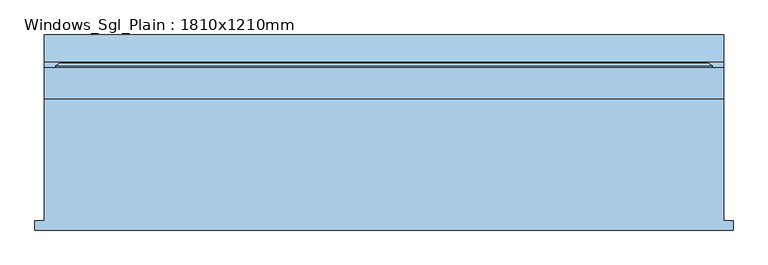
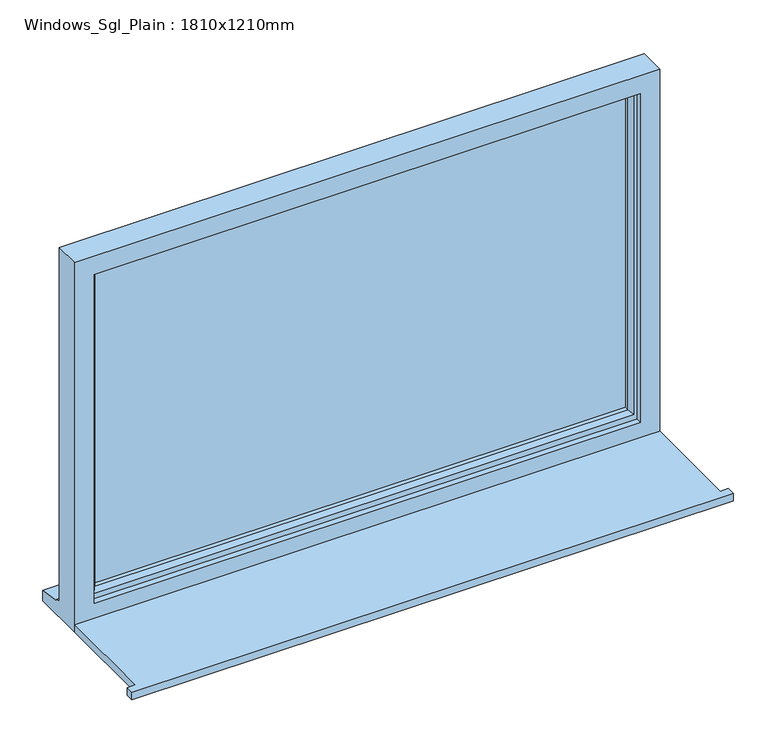
"""IFC4 building model written with IfcOpenShell, lengths in millimetres: window geometry, Windows_Sgl_Plain : 1810x1210mm."""

from ifc_helpers import new_model, si_unit, frame, origin, place, context, project, spatial, polyline, outline, extrude, faceted_brep, source, transform, mapped, element, save


def windows_sgl_plain_1810x1210mm_33e58113(model_context):
    return source(origin(), model_context, "Body", "SolidModel", [
        extrude(outline(polyline([(-930.0, -245.1434322), (-930.0, -220.1434322), (-905.0, -220.1434322), (-905.0, 104.0565678), (905.0, 104.0565678), (905.0, -220.1434322), (930.0, -220.1434322), (930.0, -245.1434322), (-930.0, -245.1434322)])), frame((0.0, 0.0, 900.0), z_axis=(0.0, 0.0, 1.0), x_axis=(1.0, 0.0, 0.0)), (0.0, 0.0, 1.0), 25.0),
        faceted_brep([(-905.0, 104.0565678, 900.0), (905.0, 104.0565678, 900.0), (905.0, 104.0565678, 2110.0), (-905.0, 104.0565678, 2110.0), (-845.0, 104.0565678, 2050.0), (845.0, 104.0565678, 2050.0), (845.0, 104.0565678, 975.0), (-845.0, 104.0565678, 975.0), (-905.0, 187.0565678, 2110.0), (-905.0, 187.0565678, 951.0), (-905.0, 202.0565678, 949.68767), (-905.0, 202.0565678, 944.7449676), (-905.0, 274.5565678, 933.8088847), (-905.0, 274.5565678, 900.0), (905.0, 187.0565678, 2110.0), (905.0, 187.0565678, 951.0), (-865.0, 187.0565678, 2070.0), (-865.0, 187.0565678, 963.0), (865.0, 187.0565678, 963.0), (865.0, 187.0565678, 2070.0), (-865.0, 122.0565678, 2070.0), (-865.0, 122.0565678, 963.0), (865.0, 122.0565678, 2070.0), (865.0, 122.0565678, 963.0), (-845.0, 122.0565678, 2050.0), (-845.0, 122.0565678, 975.0), (845.0, 122.0565678, 975.0), (845.0, 122.0565678, 2050.0), (905.0, 274.5565678, 900.0), (905.0, 274.5565678, 933.8088847), (905.0, 202.0565678, 944.7449676), (905.0, 202.0565678, 949.68767)], [[[0, 1, 2, 3], [4, 5, 6, 7]], [[0, 3, 8, 9, 10, 11, 12, 13]], [[9, 8, 14, 15], [16, 17, 18, 19]], [[17, 16, 20, 21]], [[20, 22, 23, 21], [24, 25, 26, 27]], [[24, 4, 7, 25]], [[3, 2, 14, 8]], [[16, 19, 22, 20]], [[5, 4, 24, 27]], [[15, 14, 2, 1, 28, 29, 30, 31]], [[19, 18, 23, 22]], [[5, 27, 26, 6]], [[28, 1, 0, 13]], [[29, 28, 13, 12]], [[30, 29, 12, 11]], [[31, 30, 11, 10]], [[15, 31, 10, 9]], [[21, 23, 18, 17]], [[7, 6, 26, 25]]]),
        extrude(outline(polyline([(835.0, 151.0565678), (-835.0, 151.0565678), (-835.0, 175.0565678), (835.0, 175.0565678), (835.0, 151.0565678)])), frame((0.0, 0.0, 993.0), z_axis=(0.0, 0.0, 1.0), x_axis=(1.0, 0.0, 0.0)), (0.0, 0.0, 1.0), 1047.0),
        faceted_brep([(-875.0, 187.0565678, 2080.0), (-875.0, 192.8300705, 2080.0), (-875.0, 192.8300705, 953.0), (-875.0, 187.0565678, 953.0), (-865.0, 122.0565678, 2070.0), (-865.0, 187.0565678, 2070.0), (-865.0, 187.0565678, 963.0), (-865.0, 122.0565678, 963.0), (-825.0, 136.5494677, 2030.0), (-835.1480377, 122.0565678, 2040.1480377), (-835.1480377, 122.0565678, 992.8519623), (-825.0, 136.5494677, 1003.0), (-825.0, 151.0565678, 2030.0), (-825.0, 151.0565678, 1003.0), (-835.0, 175.0565678, 2040.0), (-835.0, 151.0565678, 2040.0), (-835.0, 151.0565678, 993.0), (-835.0, 175.0565678, 993.0), (-825.0, 192.8300705, 2030.0), (-825.0, 175.0565678, 2030.0), (-825.0, 175.0565678, 1003.0), (-825.0, 192.8300705, 1003.0), (-842.4457548, 198.6035732, 2047.4457548), (-842.4457548, 198.6035732, 985.5542452), (-864.2153903, 198.6035732, 2069.2153903), (-864.2153903, 198.6035732, 963.7846097), (875.0, 192.8300705, 953.0), (875.0, 187.0565678, 953.0), (865.0, 187.0565678, 963.0), (865.0, 122.0565678, 963.0), (835.1480377, 122.0565678, 992.8519623), (825.0, 136.5494677, 1003.0), (825.0, 151.0565678, 1003.0), (835.0, 151.0565678, 993.0), (835.0, 175.0565678, 993.0), (825.0, 175.0565678, 1003.0), (825.0, 192.8300705, 1003.0), (842.4457548, 198.6035732, 985.5542452), (864.2153903, 198.6035732, 963.7846097), (875.0, 192.8300705, 2080.0), (875.0, 187.0565678, 2080.0), (865.0, 187.0565678, 2070.0), (865.0, 122.0565678, 2070.0), (835.1480377, 122.0565678, 2040.1480377), (825.0, 136.5494677, 2030.0), (825.0, 151.0565678, 2030.0), (835.0, 151.0565678, 2040.0), (835.0, 175.0565678, 2040.0), (825.0, 175.0565678, 2030.0), (825.0, 192.8300705, 2030.0), (842.4457548, 198.6035732, 2047.4457548), (864.2153903, 198.6035732, 2069.2153903)], [[[0, 1, 2, 3]], [[4, 5, 6, 7]], [[8, 9, 10, 11]], [[12, 8, 11, 13]], [[14, 15, 16, 17]], [[18, 19, 20, 21]], [[22, 18, 21, 23]], [[1, 24, 25, 2]], [[3, 2, 26, 27]], [[7, 6, 28, 29]], [[11, 10, 30, 31]], [[13, 11, 31, 32]], [[17, 16, 33, 34]], [[21, 20, 35, 36]], [[23, 21, 36, 37]], [[2, 25, 38, 26]], [[27, 26, 39, 40]], [[29, 28, 41, 42]], [[31, 30, 43, 44]], [[32, 31, 44, 45]], [[34, 33, 46, 47]], [[36, 35, 48, 49]], [[37, 36, 49, 50]], [[26, 38, 51, 39]], [[40, 39, 1, 0]], [[3, 27, 40, 0], [5, 41, 28, 6]], [[42, 41, 5, 4]], [[7, 29, 42, 4], [9, 43, 30, 10]], [[44, 43, 9, 8]], [[45, 44, 8, 12]], [[15, 46, 33, 16], [13, 32, 45, 12]], [[47, 46, 15, 14]], [[17, 34, 47, 14], [19, 48, 35, 20]], [[49, 48, 19, 18]], [[50, 49, 18, 22]], [[24, 51, 38, 25], [23, 37, 50, 22]], [[39, 51, 24, 1]]]),
    ])


if __name__ == "__main__":
    model = new_model("IFC4")
    model_context = context("Model", 3, world=origin())
    ifc_project = project(units=[si_unit("LENGTHUNIT", "METRE", prefix="MILLI")], contexts=[model_context])
    site = spatial("IfcSite", under=ifc_project)
    building = spatial("IfcBuilding", under=site)
    placement = place(None, origin())
    windows_sgl_plain_1810x1210mm_shape = windows_sgl_plain_1810x1210mm_33e58113(model_context)
    element("IfcWindow", 1, ObjectType="Windows_Sgl_Plain : 1810x1210mm", at=placement, inside=building, context=model_context, shape_type="MappedRepresentation", body=[
        mapped(windows_sgl_plain_1810x1210mm_shape, transform((0.0, 0.0, 0.0), x_axis=(1.0, 0.0, 0.0), y_axis=(0.0, 1.0, 0.0), z_axis=(0.0, 0.0, 1.0))),
    ])
    save(model, "model.ifc")

# Revit data of these elements
# Type "Windows_Sgl_Plain : 1810x1210mm"
#   Type Mark = "49"
#   Operation = "SinglePanel"
#   Construction Type Id = "SGL"
#   Manufacturer = "Revit"
#   Keynote = "L10"
#   Analytic Construction = "Large single-glazed windows"
#   Wrap Layers (Ext) from Ext = 102.5 mm
#   Wrap Layers (Int) from Ext = 177.5 mm
#   Window Board Projection = 25 mm
#   Window Board Extension = 25 mm
#   Visual Light Transmittance = 0.9
#   Solar Heat Gain Coefficient = 0.86
#   Rough Width = 1810 mm
#   Rough Height = 1210 mm
#   Height = 1210 mm
#   Width = 1810 mm
#   Heat Transfer Coefficient (U) = 5.5617 W/(m²·K)
#   Glazing Thickness = 24 mm
#   FrameOffset - External = 50 mm
#   Frame Depth = 65 mm
#   Default Head Height = 2110 mm
#   Cill Depth = 87.5 mm
#   Cavity Closer Width = 50 mm
#   Cavity Closer Offset from Ext = 102.5 mm
#   Cavity Closer Depth = 85 mm
#   Define Thermal Properties by = 1
#   Vis - Cavity Closers = yes
#   Define Thermal Properties by = 1
#   Material Trim = Window Frame
#   Material Glass = Glass
#   Material Frame = Window Frame
#   Wall Closure = (empty or 0)
# Element 1 (IfcWindow, "Windows_Sgl_Plain : 1810x1210mm")
#   Materials on its faces: "Window Frame", "Glass"
# Materials
#   "Window Frame": colour RGB 249 249 249, transparency 0, Keynote = "L10", Cost = 0
#   "Glass": class "Glass", colour RGB 0 128 192, transparency 0.9, Description = "Soda Lime Glass", Cost = 0
